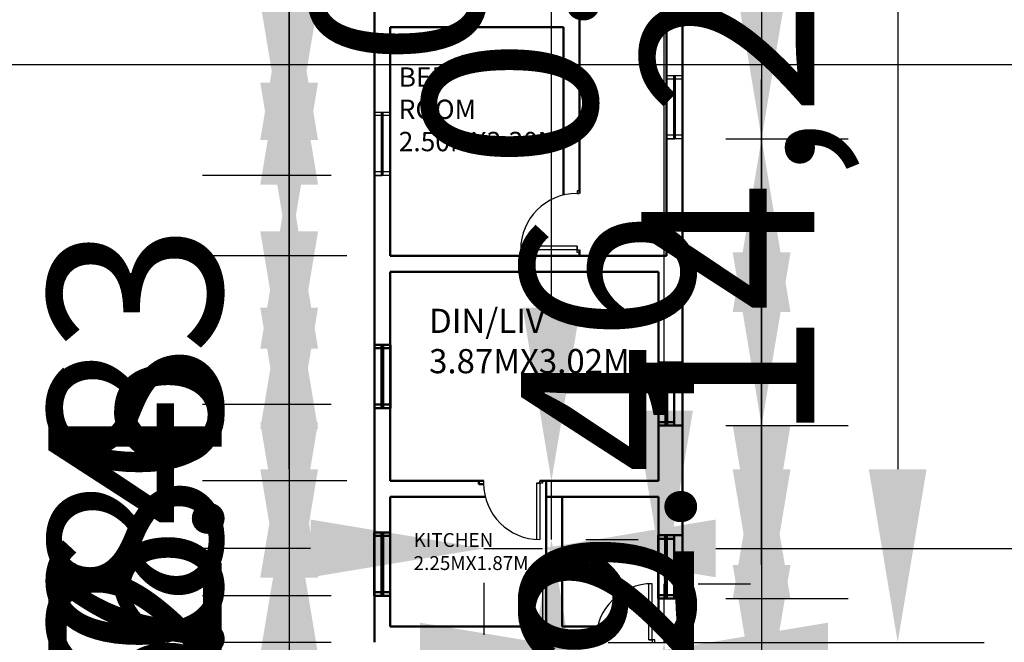
# Model space of a CAD drawing. Units: metres. Extents: x 782 to 1487, y 1262 to 7446.
# Tile 6 of 25: x 807 to 821, y 1293 to 1302. Entities that reach past the tile are written whole.
import ezdxf

# ---------------------------------------------------------------- set-up
doc = ezdxf.new("R2010")
doc.units = ezdxf.units.M
for name, color, linetype, lineweight in [('A-ANNO-DIMS', 2, 'Continuous', 18), ('A-AREA-IDEN', 3, 'Continuous', 18), ('A-DOOR', 4, 'Continuous', 25), ('A-GLAZ', 4, 'Continuous', 25), ('A-WALL', 7, 'Continuous', 50)]:
    doc.layers.add(name, color=color, linetype=linetype, lineweight=lineweight)
doc.styles.get("Standard").update_dxf_attribs({"font": 'arial.ttf'})
doc.dimstyles.new('ISO-25', dxfattribs={"dimtxt": 2.5, "dimasz": 2.5, "dimexe": 1.25, "dimexo": 0.625, "dimtad": 1, "dimtxsty": 'Standard', "dimcen": 2.5, "dimadec": 0, "dimazin": 0, "dimtfac": 1, "dimtmove": 0, "dimatfit": 3, "dimfxl": 1, "dimarcsym": 0})

# ---------------------------------------------------------------- blocks, each defined once
blk = doc.blocks.new('*D4')
at = {"layer": 'A-ANNO-DIMS', "color": 0, "lineweight": -2, "transparency": 16777216}
for p, q in [((817.205, 1307.327), (820.936, 1307.327)), ((819.686, 1304.827), (819.686, 1295.567)), ((817.205, 1293.067), (820.936, 1293.067))]:
    blk.add_line(p, q, dxfattribs=at)
at = {"layer": 'A-ANNO-DIMS', "color": 0, "transparency": 16777216}
for points in [[(819.269, 1304.827), (820.103, 1304.827), (819.686, 1307.327)], [(819.269, 1295.567), (820.103, 1295.567), (819.686, 1293.067)]]:
    blk.add_solid(points, dxfattribs=at)
at = {"layer": 'Defpoints', "color": 0, "transparency": 16777216}
for p in [(816.58, 1307.327), (816.58, 1293.067), (819.686, 1293.067)]:
    blk.add_point(p, dxfattribs=at)
at = {"layer": 'A-ANNO-DIMS', "color": 0, "transparency": 16777216, "insert": (817.558, 1300.197), "char_height": 2.5, "attachment_point": 5, "rotation": 90}
blk.add_mtext('14,26', dxfattribs=at)
blk = doc.blocks.new('DOOR-810')
for p, q in [((0.813, 0.089), (0, 0.089)), ((0.813, 0.038), (0.813, 0.089))]:
    blk.add_line(p, q)
for points in [[(0.813, 0.851), (0.846, 0.851), (0.846, 0.89), (0.813, 0.89)], [(0.813, 0.038), (0.847, 0.038), (0.847, 0), (0.813, 0)]]:
    blk.add_lwpolyline(points, close=True)
blk.add_lwpolyline([(0.813, 0.089), (0.813, 0.038), (0, 0.038)])
blk.add_arc((0.813, 0.038), 0.813, 90, 180)
blk = doc.blocks.new('DOOR-810-B')
for p, q in [((0, 0.813), (0, 0.846)), ((0.812, 0.813), (0.762, 0.813)), ((0.762, 0.813), (0.762, 0))]:
    blk.add_line(p, q)
blk.add_lwpolyline([(0.762, 0.813), (0.812, 0.813), (0.812, 0)])
blk.add_lwpolyline([(0.812, 0.813), (0.812, 0.846), (0.85, 0.846), (0.85, 0.813)], close=True)
blk.add_arc((0.812, 0.813), 0.813, 180, 270)
blk = doc.blocks.new('DOOR-810-C')
for p, q in [((0.801, 0.034), (0.801, 0.847)), ((0.851, 0.034), (0.801, 0.034))]:
    blk.add_line(p, q)
blk.add_lwpolyline([(0.801, 0.034), (0.851, 0.034), (0.851, 0.847)])
for points in [[(0.039, 0.034), (0.039, 0.002), (0, 0.002), (0, 0.034)], [(0.851, 0.034), (0.851, 0), (0.889, 0), (0.889, 0.034)]]:
    blk.add_lwpolyline(points, close=True)
blk.add_arc((0.851, 0.034), 0.813, 90, 180)
blk = doc.blocks.new('WIN-900')
for p, q in [((0, 0), (0, 0.914)), ((0, 0.914), (0.23, 0.914)), ((0.23, 0.863), (0, 0.863)), ((0.102, 0), (0.102, 0.914)), ((0.115, 0), (0.115, 0.914)), ((0.128, 0), (0.128, 0.914)), ((0.23, 0.914), (0.23, 0)), ((0.23, 0.914), (0.23, 0.863)), ((0.23, 0.051), (0, 0.051)), ((0.23, 0), (0.23, 0.051)), ((0.23, 0), (0, 0)), ((0, 0), (0.115, 0))]:
    blk.add_line(p, q)
blk = doc.blocks.new('*D22')
at = {"layer": 'A-ANNO-DIMS', "color": 0, "lineweight": -2, "transparency": 16777216}
for p, q in [((812.79, 1292.934), (810.29, 1292.934)), ((815.29, 1292.934), (816.179, 1292.934)), ((818.679, 1292.934), (848.834, 1292.934)), ((815.29, 1292.442), (815.29, 1291.684)), ((816.179, 1292.442), (816.179, 1291.684))]:
    blk.add_line(p, q, dxfattribs=at)
at = {"layer": 'A-ANNO-DIMS', "color": 0, "transparency": 16777216}
for points in [[(812.79, 1293.351), (812.79, 1292.517), (815.29, 1292.934)], [(818.679, 1293.351), (818.679, 1292.517), (816.179, 1292.934)]]:
    blk.add_solid(points, dxfattribs=at)
at = {"layer": 'Defpoints', "color": 0, "transparency": 16777216}
for p in [(815.29, 1293.067), (816.179, 1293.067), (816.179, 1292.934)]:
    blk.add_point(p, dxfattribs=at)
at = {"layer": 'A-ANNO-DIMS', "color": 0, "transparency": 16777216, "insert": (835.007, 1294.852), "char_height": 2.5, "attachment_point": 5}
blk.add_mtext('DOOR 0.89 TYP.', dxfattribs=at)
blk = doc.blocks.new('*D23')
at = {"layer": 'A-ANNO-DIMS', "color": 0, "lineweight": -2, "transparency": 16777216}
for p, q in [((816.313, 1296.414), (816.313, 1315.246)), ((816.313, 1293.067), (816.313, 1293.914)), ((816.804, 1293.914), (817.563, 1293.914)), ((816.804, 1293.067), (817.563, 1293.067)), ((816.313, 1290.567), (816.313, 1288.067))]:
    blk.add_line(p, q, dxfattribs=at)
at = {"layer": 'A-ANNO-DIMS', "color": 0, "transparency": 16777216}
for points in [[(815.896, 1296.414), (816.729, 1296.414), (816.313, 1293.914)], [(815.896, 1290.567), (816.729, 1290.567), (816.313, 1293.067)]]:
    blk.add_solid(points, dxfattribs=at)
at = {"layer": 'Defpoints', "color": 0, "transparency": 16777216}
for p in [(816.179, 1293.914), (816.313, 1293.914), (816.179, 1293.067)]:
    blk.add_point(p, dxfattribs=at)
at = {"layer": 'A-ANNO-DIMS', "color": 0, "transparency": 16777216, "insert": (814.411, 1307.08), "char_height": 2.5, "attachment_point": 5, "rotation": 90}
blk.add_mtext('0.85 TYP.', dxfattribs=at)
blk = doc.blocks.new('*D24')
at = {"layer": 'A-ANNO-DIMS', "color": 0, "lineweight": -2, "transparency": 16777216}
for p, q in [((811.209, 1294.423), (808.709, 1294.423)), ((813.709, 1294.423), (814.559, 1294.423)), ((817.059, 1294.423), (852.649, 1294.423)), ((813.709, 1293.926), (813.709, 1293.173)), ((814.559, 1293.926), (814.559, 1293.173))]:
    blk.add_line(p, q, dxfattribs=at)
at = {"layer": 'A-ANNO-DIMS', "color": 0, "transparency": 16777216}
for points in [[(811.209, 1294.84), (811.209, 1294.006), (813.709, 1294.423)], [(817.059, 1294.84), (817.059, 1294.006), (814.559, 1294.423)]]:
    blk.add_solid(points, dxfattribs=at)
at = {"layer": 'Defpoints', "color": 0, "transparency": 16777216}
for p in [(813.709, 1294.551), (814.559, 1294.551), (814.559, 1294.423)]:
    blk.add_point(p, dxfattribs=at)
at = {"layer": 'A-ANNO-DIMS', "color": 0, "transparency": 16777216, "insert": (836.104, 1296.342), "char_height": 2.5, "attachment_point": 5}
blk.add_mtext('DOOR D2 0.85 TYP.', dxfattribs=at)
blk = doc.blocks.new('*D25')
at = {"layer": 'A-ANNO-DIMS', "color": 0, "lineweight": -2, "transparency": 16777216}
for p, q in [((814.687, 1297.897), (814.687, 1316.729)), ((814.687, 1294.551), (814.687, 1295.397)), ((815.184, 1295.397), (815.937, 1295.397)), ((815.184, 1294.551), (815.937, 1294.551)), ((814.687, 1292.051), (814.687, 1289.551))]:
    blk.add_line(p, q, dxfattribs=at)
at = {"layer": 'A-ANNO-DIMS', "color": 0, "transparency": 16777216}
for points in [[(814.27, 1297.897), (815.103, 1297.897), (814.687, 1295.397)], [(814.27, 1292.051), (815.103, 1292.051), (814.687, 1294.551)]]:
    blk.add_solid(points, dxfattribs=at)
at = {"layer": 'Defpoints', "color": 0, "transparency": 16777216}
for p in [(814.559, 1295.397), (814.687, 1295.397), (814.559, 1294.551)]:
    blk.add_point(p, dxfattribs=at)
at = {"layer": 'A-ANNO-DIMS', "color": 0, "transparency": 16777216, "insert": (812.785, 1308.563), "char_height": 2.5, "attachment_point": 5, "rotation": 90}
blk.add_mtext('0.85 TYP.', dxfattribs=at)
blk = doc.blocks.new('*D26')
at = {"layer": 'A-ANNO-DIMS', "color": 0, "lineweight": -2, "transparency": 16777216}
for p, q in [((828.33, 1303.223), (828.33, 1342.718)), ((828.33, 1299.809), (828.33, 1300.723)), ((828.818, 1300.723), (829.58, 1300.723)), ((828.818, 1299.809), (829.58, 1299.809)), ((828.33, 1297.309), (828.33, 1294.809))]:
    blk.add_line(p, q, dxfattribs=at)
at = {"layer": 'A-ANNO-DIMS', "color": 0, "transparency": 16777216}
for points in [[(827.913, 1303.223), (828.747, 1303.223), (828.33, 1300.723)], [(827.913, 1297.309), (828.747, 1297.309), (828.33, 1299.809)]]:
    blk.add_solid(points, dxfattribs=at)
at = {"layer": 'Defpoints', "color": 0, "transparency": 16777216}
for p in [(828.193, 1300.723), (828.33, 1300.723), (828.193, 1299.809)]:
    blk.add_point(p, dxfattribs=at)
at = {"layer": 'A-ANNO-DIMS', "color": 0, "transparency": 16777216, "insert": (826.412, 1324.22), "char_height": 2.5, "attachment_point": 5, "rotation": 90}
blk.add_mtext('WINDOW W 0.91 TYP.', dxfattribs=at)
blk = doc.blocks.new('*D30')
at = {"layer": 'A-ANNO-DIMS', "color": 0, "lineweight": -2, "transparency": 16777216}
for p, q in [((792.059, 1301.411), (789.559, 1301.411)), ((794.559, 1301.411), (794.946, 1301.411)), ((797.446, 1301.411), (832.354, 1301.411)), ((794.559, 1300.844), (794.559, 1300.161)), ((794.946, 1300.844), (794.946, 1300.161))]:
    blk.add_line(p, q, dxfattribs=at)
at = {"layer": 'A-ANNO-DIMS', "color": 0, "transparency": 16777216}
for points in [[(792.059, 1301.827), (792.059, 1300.994), (794.559, 1301.411)], [(797.446, 1301.827), (797.446, 1300.994), (794.946, 1301.411)]]:
    blk.add_solid(points, dxfattribs=at)
at = {"layer": 'Defpoints', "color": 0, "transparency": 16777216}
for p in [(794.559, 1301.469), (794.946, 1301.469), (794.946, 1301.411)]:
    blk.add_point(p, dxfattribs=at)
at = {"layer": 'A-ANNO-DIMS', "color": 0, "transparency": 16777216, "insert": (816.15, 1303.33), "char_height": 2.5, "attachment_point": 5}
blk.add_mtext('COLUMN 0.39 TYP.', dxfattribs=at)
blk = doc.blocks.new('*D48')
at = {"layer": 'A-ANNO-DIMS', "color": 0, "lineweight": -2, "transparency": 16777216}
for p, q in [((795.937, 1293.455), (795.937, 1287.89)), ((794.559, 1292.035), (794.559, 1287.89)), ((792.059, 1289.14), (789.559, 1289.14)), ((794.559, 1289.14), (795.937, 1289.14)), ((798.437, 1289.14), (808.45, 1289.14))]:
    blk.add_line(p, q, dxfattribs=at)
at = {"layer": 'A-ANNO-DIMS', "color": 0, "transparency": 16777216}
for points in [[(792.059, 1289.557), (792.059, 1288.724), (794.559, 1289.14)], [(798.437, 1289.557), (798.437, 1288.724), (795.937, 1289.14)]]:
    blk.add_solid(points, dxfattribs=at)
at = {"layer": 'Defpoints', "color": 0, "transparency": 16777216}
for p in [(795.937, 1294.08), (794.559, 1292.66), (795.937, 1289.14)]:
    blk.add_point(p, dxfattribs=at)
at = {"layer": 'A-ANNO-DIMS', "color": 0, "transparency": 16777216, "insert": (804.694, 1291.043), "char_height": 2.5, "attachment_point": 5}
blk.add_mtext('1.38', dxfattribs=at)
blk = doc.blocks.new('*D53')
at = {"layer": 'A-ANNO-DIMS', "color": 0, "lineweight": -2, "transparency": 16777216}
for p, q in [((810.9, 1309.827), (810.9, 1312.327)), ((811.505, 1307.327), (809.65, 1307.327)), ((810.9, 1307.327), (810.9, 1304.697)), ((811.735, 1304.697), (809.65, 1304.697)), ((810.9, 1302.197), (810.9, 1291.911))]:
    blk.add_line(p, q, dxfattribs=at)
at = {"layer": 'A-ANNO-DIMS', "color": 0, "transparency": 16777216}
for points in [[(810.483, 1309.827), (811.317, 1309.827), (810.9, 1307.327)], [(810.483, 1302.197), (811.317, 1302.197), (810.9, 1304.697)]]:
    blk.add_solid(points, dxfattribs=at)
at = {"layer": 'Defpoints', "color": 0, "transparency": 16777216}
for p in [(812.13, 1307.327), (810.9, 1304.697), (812.36, 1304.697)]:
    blk.add_point(p, dxfattribs=at)
at = {"layer": 'A-ANNO-DIMS', "color": 0, "transparency": 16777216, "insert": (808.998, 1295.804), "char_height": 2.5, "attachment_point": 5, "rotation": 90}
blk.add_mtext('2.63', dxfattribs=at)
blk = doc.blocks.new('*D54')
at = {"layer": 'A-ANNO-DIMS', "color": 0, "lineweight": -2, "transparency": 16777216}
for p, q in [((810.9, 1307.197), (810.9, 1309.697)), ((811.735, 1304.697), (809.65, 1304.697)), ((810.9, 1304.697), (810.9, 1302.822)), ((811.503, 1302.822), (809.65, 1302.822)), ((810.9, 1300.322), (810.9, 1290.308))]:
    blk.add_line(p, q, dxfattribs=at)
at = {"layer": 'A-ANNO-DIMS', "color": 0, "transparency": 16777216}
for points in [[(810.483, 1307.197), (811.317, 1307.197), (810.9, 1304.697)], [(810.483, 1300.322), (811.317, 1300.322), (810.9, 1302.822)]]:
    blk.add_solid(points, dxfattribs=at)
at = {"layer": 'Defpoints', "color": 0, "transparency": 16777216}
for p in [(812.36, 1304.697), (810.9, 1302.822), (812.128, 1302.822)]:
    blk.add_point(p, dxfattribs=at)
at = {"layer": 'A-ANNO-DIMS', "color": 0, "transparency": 16777216, "insert": (808.999, 1294.065), "char_height": 2.5, "attachment_point": 5, "rotation": 90}
blk.add_mtext('1.88', dxfattribs=at)
blk = doc.blocks.new('*D55')
at = {"layer": 'A-ANNO-DIMS', "color": 0, "lineweight": -2, "transparency": 16777216}
for p, q in [((810.9, 1305.322), (810.9, 1307.822)), ((811.503, 1302.822), (809.65, 1302.822)), ((810.9, 1302.822), (810.9, 1302.177)), ((811.735, 1302.177), (809.65, 1302.177)), ((810.9, 1299.677), (810.9, 1289.444))]:
    blk.add_line(p, q, dxfattribs=at)
at = {"layer": 'A-ANNO-DIMS', "color": 0, "transparency": 16777216}
for points in [[(810.483, 1305.322), (811.317, 1305.322), (810.9, 1302.822)], [(810.483, 1299.677), (811.317, 1299.677), (810.9, 1302.177)]]:
    blk.add_solid(points, dxfattribs=at)
at = {"layer": 'Defpoints', "color": 0, "transparency": 16777216}
for p in [(812.128, 1302.822), (810.9, 1302.177), (812.36, 1302.177)]:
    blk.add_point(p, dxfattribs=at)
at = {"layer": 'A-ANNO-DIMS', "color": 0, "transparency": 16777216, "insert": (808.999, 1293.311), "char_height": 2.5, "attachment_point": 5, "rotation": 90}
blk.add_mtext('0.64', dxfattribs=at)
blk = doc.blocks.new('*D56')
at = {"layer": 'A-ANNO-DIMS', "color": 0, "lineweight": -2, "transparency": 16777216}
for p, q in [((810.9, 1304.677), (810.9, 1307.177)), ((811.735, 1302.177), (809.65, 1302.177)), ((810.9, 1302.177), (810.9, 1299.809)), ((811.505, 1299.809), (809.65, 1299.809)), ((810.9, 1297.309), (810.9, 1287.022))]:
    blk.add_line(p, q, dxfattribs=at)
at = {"layer": 'A-ANNO-DIMS', "color": 0, "transparency": 16777216}
for points in [[(810.483, 1304.677), (811.317, 1304.677), (810.9, 1302.177)], [(810.483, 1297.309), (811.317, 1297.309), (810.9, 1299.809)]]:
    blk.add_solid(points, dxfattribs=at)
at = {"layer": 'Defpoints', "color": 0, "transparency": 16777216}
for p in [(812.36, 1302.177), (810.9, 1299.809), (812.13, 1299.809)]:
    blk.add_point(p, dxfattribs=at)
at = {"layer": 'A-ANNO-DIMS', "color": 0, "transparency": 16777216, "insert": (808.998, 1290.916), "char_height": 2.5, "attachment_point": 5, "rotation": 90}
blk.add_mtext('2.37', dxfattribs=at)
blk = doc.blocks.new('*D57')
at = {"layer": 'A-ANNO-DIMS', "color": 0, "lineweight": -2, "transparency": 16777216}
for p, q in [((810.9, 1302.309), (810.9, 1304.809)), ((811.505, 1299.809), (809.65, 1299.809)), ((810.9, 1299.809), (810.9, 1298.647)), ((811.735, 1298.647), (809.65, 1298.647)), ((810.9, 1296.147), (810.9, 1286.141))]:
    blk.add_line(p, q, dxfattribs=at)
at = {"layer": 'A-ANNO-DIMS', "color": 0, "transparency": 16777216}
for points in [[(810.483, 1302.309), (811.317, 1302.309), (810.9, 1299.809)], [(810.483, 1296.147), (811.317, 1296.147), (810.9, 1298.647)]]:
    blk.add_solid(points, dxfattribs=at)
at = {"layer": 'Defpoints', "color": 0, "transparency": 16777216}
for p in [(812.13, 1299.809), (810.9, 1298.647), (812.36, 1298.647)]:
    blk.add_point(p, dxfattribs=at)
at = {"layer": 'A-ANNO-DIMS', "color": 0, "transparency": 16777216, "insert": (808.999, 1289.894), "char_height": 2.5, "attachment_point": 5, "rotation": 90}
blk.add_mtext('1.16', dxfattribs=at)
blk = doc.blocks.new('*D58')
at = {"layer": 'A-ANNO-DIMS', "color": 0, "lineweight": -2, "transparency": 16777216}
for p, q in [((810.9, 1301.147), (810.9, 1303.647)), ((811.735, 1298.647), (809.65, 1298.647)), ((810.9, 1298.647), (810.9, 1296.5)), ((811.507, 1296.5), (809.65, 1296.5)), ((810.9, 1294), (810.9, 1281.772))]:
    blk.add_line(p, q, dxfattribs=at)
at = {"layer": 'A-ANNO-DIMS', "color": 0, "transparency": 16777216}
for points in [[(810.483, 1301.147), (811.317, 1301.147), (810.9, 1298.647)], [(810.483, 1294), (811.317, 1294), (810.9, 1296.5)]]:
    blk.add_solid(points, dxfattribs=at)
at = {"layer": 'Defpoints', "color": 0, "transparency": 16777216}
for p in [(812.36, 1298.647), (810.9, 1296.5), (812.132, 1296.5)]:
    blk.add_point(p, dxfattribs=at)
at = {"layer": 'A-ANNO-DIMS', "color": 0, "transparency": 16777216, "insert": (809.02, 1286.636), "char_height": 2.5, "attachment_point": 5, "rotation": 90}
blk.add_mtext('2.147', dxfattribs=at)
blk = doc.blocks.new('*D59')
at = {"layer": 'A-ANNO-DIMS', "color": 0, "lineweight": -2, "transparency": 16777216}
for p, q in [((810.9, 1299), (810.9, 1301.5)), ((811.507, 1296.5), (809.65, 1296.5)), ((810.9, 1296.5), (810.9, 1295.397)), ((811.735, 1295.397), (809.65, 1295.397)), ((810.9, 1292.897), (810.9, 1280.947))]:
    blk.add_line(p, q, dxfattribs=at)
at = {"layer": 'A-ANNO-DIMS', "color": 0, "transparency": 16777216}
for points in [[(810.483, 1299), (811.317, 1299), (810.9, 1296.5)], [(810.483, 1292.897), (811.317, 1292.897), (810.9, 1295.397)]]:
    blk.add_solid(points, dxfattribs=at)
at = {"layer": 'Defpoints', "color": 0, "transparency": 16777216}
for p in [(812.132, 1296.5), (810.9, 1295.397), (812.36, 1295.397)]:
    blk.add_point(p, dxfattribs=at)
at = {"layer": 'A-ANNO-DIMS', "color": 0, "transparency": 16777216, "insert": (808.998, 1285.672), "char_height": 2.5, "attachment_point": 5, "rotation": 90}
blk.add_mtext('1.103', dxfattribs=at)
blk = doc.blocks.new('*D60')
at = {"layer": 'A-ANNO-DIMS', "color": 0, "lineweight": -2, "transparency": 16777216}
for p, q in [((810.9, 1297.897), (810.9, 1300.397)), ((811.735, 1295.397), (809.65, 1295.397)), ((810.9, 1295.397), (810.9, 1293.74)), ((811.505, 1293.74), (809.65, 1293.74)), ((810.9, 1291.24), (810.9, 1281.233))]:
    blk.add_line(p, q, dxfattribs=at)
at = {"layer": 'A-ANNO-DIMS', "color": 0, "transparency": 16777216}
for points in [[(810.483, 1297.897), (811.317, 1297.897), (810.9, 1295.397)], [(810.483, 1291.24), (811.317, 1291.24), (810.9, 1293.74)]]:
    blk.add_solid(points, dxfattribs=at)
at = {"layer": 'Defpoints', "color": 0, "transparency": 16777216}
for p in [(812.36, 1295.397), (810.9, 1293.74), (812.13, 1293.74)]:
    blk.add_point(p, dxfattribs=at)
at = {"layer": 'A-ANNO-DIMS', "color": 0, "transparency": 16777216, "insert": (808.999, 1284.987), "char_height": 2.5, "attachment_point": 5, "rotation": 90}
blk.add_mtext('1.66', dxfattribs=at)
blk = doc.blocks.new('*D61')
at = {"layer": 'A-ANNO-DIMS', "color": 0, "lineweight": -2, "transparency": 16777216}
for p, q in [((810.9, 1296.24), (810.9, 1298.74)), ((811.505, 1293.74), (809.65, 1293.74)), ((810.9, 1293.74), (810.9, 1293.067)), ((811.505, 1293.067), (809.65, 1293.067)), ((810.9, 1290.567), (810.9, 1280.324))]:
    blk.add_line(p, q, dxfattribs=at)
at = {"layer": 'A-ANNO-DIMS', "color": 0, "transparency": 16777216}
for points in [[(810.483, 1296.24), (811.317, 1296.24), (810.9, 1293.74)], [(810.483, 1290.567), (811.317, 1290.567), (810.9, 1293.067)]]:
    blk.add_solid(points, dxfattribs=at)
at = {"layer": 'Defpoints', "color": 0, "transparency": 16777216}
for p in [(812.13, 1293.74), (810.9, 1293.067), (812.13, 1293.067)]:
    blk.add_point(p, dxfattribs=at)
at = {"layer": 'A-ANNO-DIMS', "color": 0, "transparency": 16777216, "insert": (808.999, 1284.195), "char_height": 2.5, "attachment_point": 5, "rotation": 90}
blk.add_mtext('0.67', dxfattribs=at)
blk = doc.blocks.new('*D62')
at = {"layer": 'A-ANNO-DIMS', "color": 0, "lineweight": -2, "transparency": 16777216}
for p, q in [((810.9, 1295.567), (810.9, 1298.067)), ((811.505, 1293.067), (809.65, 1293.067)), ((810.9, 1293.067), (810.9, 1290.305)), ((811.505, 1290.305), (809.65, 1290.305)), ((810.9, 1287.805), (810.9, 1275.602))]:
    blk.add_line(p, q, dxfattribs=at)
at = {"layer": 'A-ANNO-DIMS', "color": 0, "transparency": 16777216}
for points in [[(810.483, 1295.567), (811.317, 1295.567), (810.9, 1293.067)], [(810.483, 1287.805), (811.317, 1287.805), (810.9, 1290.305)]]:
    blk.add_solid(points, dxfattribs=at)
at = {"layer": 'Defpoints', "color": 0, "transparency": 16777216}
for p in [(812.13, 1293.067), (810.9, 1290.305), (812.13, 1290.305)]:
    blk.add_point(p, dxfattribs=at)
at = {"layer": 'A-ANNO-DIMS', "color": 0, "transparency": 16777216, "insert": (808.999, 1280.454), "char_height": 2.5, "attachment_point": 5, "rotation": 90}
blk.add_mtext('2.762', dxfattribs=at)
blk = doc.blocks.new('*D63')
at = {"layer": 'A-ANNO-DIMS', "color": 0, "lineweight": -2, "transparency": 16777216}
for p, q in [((817.721, 1309.827), (817.721, 1312.327)), ((817.205, 1307.327), (818.971, 1307.327)), ((817.721, 1307.327), (817.721, 1304.867)), ((817.205, 1304.867), (818.971, 1304.867)), ((817.721, 1302.367), (817.721, 1292.082))]:
    blk.add_line(p, q, dxfattribs=at)
at = {"layer": 'A-ANNO-DIMS', "color": 0, "transparency": 16777216}
for points in [[(817.304, 1309.827), (818.138, 1309.827), (817.721, 1307.327)], [(817.304, 1302.367), (818.138, 1302.367), (817.721, 1304.867)]]:
    blk.add_solid(points, dxfattribs=at)
at = {"layer": 'Defpoints', "color": 0, "transparency": 16777216}
for p in [(816.58, 1307.327), (816.58, 1304.867), (817.721, 1304.867)]:
    blk.add_point(p, dxfattribs=at)
at = {"layer": 'A-ANNO-DIMS', "color": 0, "transparency": 16777216, "insert": (815.82, 1295.974), "char_height": 2.5, "attachment_point": 5, "rotation": 90}
blk.add_mtext('2.46', dxfattribs=at)
blk = doc.blocks.new('*D64')
at = {"layer": 'A-ANNO-DIMS', "color": 0, "lineweight": -2, "transparency": 16777216}
for p, q in [((817.721, 1307.367), (817.721, 1309.867)), ((817.205, 1304.867), (818.971, 1304.867)), ((817.721, 1304.867), (817.721, 1300.338)), ((817.206, 1300.338), (818.971, 1300.338)), ((817.721, 1297.838), (817.721, 1285.546))]:
    blk.add_line(p, q, dxfattribs=at)
at = {"layer": 'A-ANNO-DIMS', "color": 0, "transparency": 16777216}
for points in [[(817.304, 1307.367), (818.138, 1307.367), (817.721, 1304.867)], [(817.304, 1297.838), (818.138, 1297.838), (817.721, 1300.338)]]:
    blk.add_solid(points, dxfattribs=at)
at = {"layer": 'Defpoints', "color": 0, "transparency": 16777216}
for p in [(816.58, 1304.867), (816.581, 1300.338), (817.721, 1300.338)]:
    blk.add_point(p, dxfattribs=at)
at = {"layer": 'A-ANNO-DIMS', "color": 0, "transparency": 16777216, "insert": (815.82, 1290.442), "char_height": 2.5, "attachment_point": 5, "rotation": 90}
blk.add_mtext('4.529', dxfattribs=at)
blk = doc.blocks.new('*D65')
at = {"layer": 'A-ANNO-DIMS', "color": 0, "lineweight": -2, "transparency": 16777216}
for p, q in [((817.721, 1302.838), (817.721, 1305.338)), ((817.206, 1300.338), (818.971, 1300.338)), ((817.721, 1300.338), (817.721, 1296.196)), ((817.205, 1296.196), (818.971, 1296.196)), ((817.721, 1293.696), (817.721, 1281.435))]:
    blk.add_line(p, q, dxfattribs=at)
at = {"layer": 'A-ANNO-DIMS', "color": 0, "transparency": 16777216}
for points in [[(817.304, 1302.838), (818.138, 1302.838), (817.721, 1300.338)], [(817.304, 1293.696), (818.138, 1293.696), (817.721, 1296.196)]]:
    blk.add_solid(points, dxfattribs=at)
at = {"layer": 'Defpoints', "color": 0, "transparency": 16777216}
for p in [(816.581, 1300.338), (816.58, 1296.196), (817.721, 1296.196)]:
    blk.add_point(p, dxfattribs=at)
at = {"layer": 'A-ANNO-DIMS', "color": 0, "transparency": 16777216, "insert": (815.841, 1286.315), "char_height": 2.5, "attachment_point": 5, "rotation": 90}
blk.add_mtext('4.142', dxfattribs=at)
blk = doc.blocks.new('*D66')
at = {"layer": 'A-ANNO-DIMS', "color": 0, "lineweight": -2, "transparency": 16777216}
for p, q in [((817.721, 1298.696), (817.721, 1301.196)), ((817.205, 1296.196), (818.971, 1296.196)), ((817.721, 1296.196), (817.721, 1293.699)), ((817.205, 1293.699), (818.971, 1293.699)), ((817.721, 1291.199), (817.721, 1280.921))]:
    blk.add_line(p, q, dxfattribs=at)
at = {"layer": 'A-ANNO-DIMS', "color": 0, "transparency": 16777216}
for points in [[(817.304, 1298.696), (818.138, 1298.696), (817.721, 1296.196)], [(817.304, 1291.199), (818.138, 1291.199), (817.721, 1293.699)]]:
    blk.add_solid(points, dxfattribs=at)
at = {"layer": 'Defpoints', "color": 0, "transparency": 16777216}
for p in [(816.58, 1296.196), (816.58, 1293.699), (817.721, 1293.699)]:
    blk.add_point(p, dxfattribs=at)
at = {"layer": 'A-ANNO-DIMS', "color": 0, "transparency": 16777216, "insert": (815.82, 1284.81), "char_height": 2.5, "attachment_point": 5, "rotation": 90}
blk.add_mtext('2.50', dxfattribs=at)
blk = doc.blocks.new('*D67')
at = {"layer": 'A-ANNO-DIMS', "color": 0, "lineweight": -2, "transparency": 16777216}
for p, q in [((817.721, 1296.199), (817.721, 1298.699)), ((817.205, 1293.699), (818.971, 1293.699)), ((817.721, 1293.699), (817.721, 1293.067)), ((817.205, 1293.067), (818.971, 1293.067)), ((817.721, 1290.567), (817.721, 1278.407))]:
    blk.add_line(p, q, dxfattribs=at)
at = {"layer": 'A-ANNO-DIMS', "color": 0, "transparency": 16777216}
for points in [[(817.304, 1296.199), (818.138, 1296.199), (817.721, 1293.699)], [(817.304, 1290.567), (818.138, 1290.567), (817.721, 1293.067)]]:
    blk.add_solid(points, dxfattribs=at)
at = {"layer": 'Defpoints', "color": 0, "transparency": 16777216}
for p in [(816.58, 1293.699), (816.58, 1293.067), (817.721, 1293.067)]:
    blk.add_point(p, dxfattribs=at)
at = {"layer": 'A-ANNO-DIMS', "color": 0, "transparency": 16777216, "insert": (815.819, 1283.237), "char_height": 2.5, "attachment_point": 5, "rotation": 90}
blk.add_mtext('0.632', dxfattribs=at)
blk = doc.blocks.new('*D68')
at = {"layer": 'A-ANNO-DIMS', "color": 0, "lineweight": -2, "transparency": 16777216}
for p, q in [((817.721, 1295.567), (817.721, 1298.067)), ((815.508, 1293.067), (818.971, 1293.067)), ((817.721, 1293.067), (817.721, 1291.686)), ((815.508, 1291.686), (818.971, 1291.686)), ((817.721, 1289.186), (817.721, 1277.718))]:
    blk.add_line(p, q, dxfattribs=at)
at = {"layer": 'A-ANNO-DIMS', "color": 0, "transparency": 16777216}
for points in [[(817.304, 1295.567), (818.138, 1295.567), (817.721, 1293.067)], [(817.304, 1289.186), (818.138, 1289.186), (817.721, 1291.686)]]:
    blk.add_solid(points, dxfattribs=at)
at = {"layer": 'Defpoints', "color": 0, "transparency": 16777216}
for p in [(814.883, 1293.067), (814.883, 1291.686), (817.721, 1291.686)]:
    blk.add_point(p, dxfattribs=at)
at = {"layer": 'A-ANNO-DIMS', "color": 0, "transparency": 16777216, "insert": (815.819, 1282.202), "char_height": 2.5, "attachment_point": 5, "rotation": 90}
blk.add_mtext('1.381', dxfattribs=at)
blk = doc.blocks.new('*D69')
at = {"layer": 'A-ANNO-DIMS', "color": 0, "lineweight": -2, "transparency": 16777216}
for p, q in [((817.721, 1294.186), (817.721, 1296.686)), ((815.508, 1291.686), (818.971, 1291.686)), ((817.721, 1291.686), (817.721, 1290.305)), ((815.508, 1290.305), (818.971, 1290.305)), ((817.721, 1287.805), (817.721, 1276.337))]:
    blk.add_line(p, q, dxfattribs=at)
at = {"layer": 'A-ANNO-DIMS', "color": 0, "transparency": 16777216}
for points in [[(817.304, 1294.186), (818.138, 1294.186), (817.721, 1291.686)], [(817.304, 1287.805), (818.138, 1287.805), (817.721, 1290.305)]]:
    blk.add_solid(points, dxfattribs=at)
at = {"layer": 'Defpoints', "color": 0, "transparency": 16777216}
for p in [(814.883, 1291.686), (814.883, 1290.305), (817.721, 1290.305)]:
    blk.add_point(p, dxfattribs=at)
at = {"layer": 'A-ANNO-DIMS', "color": 0, "transparency": 16777216, "insert": (815.819, 1280.821), "char_height": 2.5, "attachment_point": 5, "rotation": 90}
blk.add_mtext('1.381', dxfattribs=at)

msp = doc.modelspace()

# ---------------------------------------------------------------- linework, layer by layer
at = {"layer": 'A-WALL'}
for p, q in [((816.58, 1303.3374), (816.58, 1293.0674)), ((816.35, 1303.1074), (816.35, 1298.6474)), ((812.13, 1298.6474), (812.13, 1302.1774)), ((815.09, 1302.1774), (815.09, 1299.5481)), ((812.36, 1298.6474), (812.36, 1301.9474)), ((812.36, 1301.9474), (814.86, 1301.9474)), ((814.86, 1301.9474), (814.86, 1299.5248)), ((815.09, 1298.736), (815.09, 1298.6474)), ((812.13, 1295.3974), (812.13, 1298.6474)), ((812.36, 1298.6474), (816.23, 1298.6474)), ((815.09, 1298.6474), (815.09, 1298.6982)), ((816.35, 1298.6474), (816.23, 1298.6474)), ((812.36, 1295.3974), (812.36, 1298.4174)), ((812.36, 1298.4174), (816.23, 1298.4174)), ((812.36, 1298.4174), (816.23, 1298.4174)), ((816.23, 1298.4174), (816.23, 1295.3974)), ((812.1317, 1296.4496), (812.1317, 1297.3636)), ((812.1317, 1297.3636), (812.3617, 1297.3636)), ((812.3617, 1297.3128), (812.1317, 1297.3128)), ((812.234, 1296.4496), (812.234, 1297.3636)), ((812.2467, 1296.4496), (812.2467, 1297.3636)), ((812.2594, 1296.4496), (812.2594, 1297.3636)), ((812.3617, 1297.3636), (812.3617, 1296.4496)), ((812.3617, 1297.3636), (812.3617, 1297.3128)), ((816.2301, 1296.196), (816.2301, 1297.11)), ((816.2301, 1297.11), (816.4601, 1297.11)), ((816.4601, 1297.0592), (816.2301, 1297.0592)), ((816.3324, 1296.196), (816.3324, 1297.11)), ((816.3451, 1296.196), (816.3451, 1297.11)), ((816.3578, 1296.196), (816.3578, 1297.11)), ((816.4601, 1297.11), (816.4601, 1296.196)), ((816.4601, 1297.11), (816.4601, 1297.0592)), ((816.4601, 1297.11), (816.58, 1297.11)), ((816.58, 1297.11), (816.58, 1296.196)), ((812.3617, 1296.5004), (812.1317, 1296.5004)), ((812.3617, 1296.4496), (812.3617, 1296.5004)), ((812.3617, 1296.4496), (812.1317, 1296.4496)), ((812.1317, 1296.4496), (812.2467, 1296.4496)), ((816.4601, 1296.2468), (816.2301, 1296.2468)), ((816.4601, 1296.196), (816.2301, 1296.196)), ((816.2301, 1296.196), (816.3451, 1296.196)), ((816.4601, 1296.196), (816.4601, 1296.2468)), ((816.58, 1296.196), (816.4601, 1296.196)), ((812.13, 1295.3974), (812.13, 1293.0674)), ((813.7093, 1295.3974), (812.36, 1295.3974)), ((813.7093, 1295.3974), (812.36, 1295.3974)), ((813.7086, 1295.3974), (813.6406, 1295.3974)), ((813.6406, 1295.3974), (813.6406, 1295.3502)), ((813.6406, 1295.3502), (813.7087, 1295.3502)), ((814.61, 1295.3974), (814.5214, 1295.3974)), ((816.23, 1295.3974), (814.5214, 1295.3974)), ((814.61, 1295.3974), (814.5592, 1295.3974)), ((814.61, 1295.1674), (814.61, 1295.3974)), ((812.36, 1295.1674), (812.36, 1293.2974)), ((813.7326, 1295.1674), (812.36, 1295.1674)), ((813.7326, 1295.1674), (812.36, 1295.1674)), ((814.61, 1293.2974), (814.61, 1295.1674)), ((816.23, 1295.1674), (814.61, 1295.1674)), ((814.84, 1293.2974), (814.84, 1295.1674)), ((816.23, 1293.2974), (816.23, 1295.1674)), ((812.1297, 1293.7402), (812.1297, 1294.6542)), ((812.1297, 1294.6542), (812.3597, 1294.6542)), ((812.232, 1293.7402), (812.232, 1294.6542)), ((812.2447, 1293.7402), (812.2447, 1294.6542)), ((812.2574, 1293.7402), (812.2574, 1294.6542)), ((812.3597, 1294.6542), (812.3597, 1293.7402)), ((812.3597, 1294.6542), (812.3597, 1294.6034)), ((816.2268, 1293.6994), (816.2268, 1294.6134)), ((816.2268, 1294.6134), (816.4568, 1294.6134)), ((816.3291, 1293.6994), (816.3291, 1294.6134)), ((816.3418, 1293.6994), (816.3418, 1294.6134)), ((816.3545, 1293.6994), (816.3545, 1294.6134)), ((816.4568, 1294.6134), (816.4568, 1293.6994)), ((816.4568, 1294.6134), (816.4568, 1294.5626)), ((816.4568, 1294.6134), (816.58, 1294.6134)), ((816.58, 1294.6134), (816.58, 1293.6994)), ((812.3597, 1294.6034), (812.1297, 1294.6034)), ((816.4568, 1294.5626), (816.2268, 1294.5626)), ((812.3597, 1293.791), (812.1297, 1293.791)), ((812.3597, 1293.7402), (812.3597, 1293.791)), ((812.3597, 1293.7402), (812.1297, 1293.7402)), ((812.1297, 1293.7402), (812.2447, 1293.7402)), ((816.4568, 1293.7502), (816.2268, 1293.7502)), ((816.4568, 1293.6994), (816.2268, 1293.6994)), ((816.2268, 1293.6994), (816.3418, 1293.6994)), ((816.4568, 1293.6994), (816.4568, 1293.7502)), ((816.58, 1293.6994), (816.4568, 1293.6994)), ((812.36, 1293.2974), (814.61, 1293.2974)), ((814.84, 1293.2974), (815.3526, 1293.2974)), ((816.1414, 1293.2974), (816.23, 1293.2974))]:
    msp.add_line(p, q, dxfattribs=at)

# ---------------------------------------------------------------- block references
at = {"layer": 'A-DOOR'}
for name, p in [('DOOR-810', (814.243, 1298.698)), ('DOOR-810-B', (813.709, 1294.551)), ('DOOR-810-C', (815.29, 1293.067))]:
    msp.add_blockref(name, p, dxfattribs=at)
at = {"layer": 'A-GLAZ'}
for p in [(816.351, 1300.338), (812.13, 1299.809)]:
    msp.add_blockref('WIN-900', p, dxfattribs=at)

# ---------------------------------------------------------------- texts
at = {"layer": 'A-AREA-IDEN', "attachment_point": 1}
for s, width, gutter_width, insert, char_height in [('BED ROOM\\P2.50MX3.30M', 0.64421, 6.9836, (812.4812, 1301.3688), 0.279342), ('DIN/LIV\\P3.87MX3.02M', 0.805163, 8.7284, (812.9207, 1297.8835), 0.349134), ('{\\H0.4x;\\PKITCHEN\\P2.25MX1.87M}', 1.153085, 12.5, (812.6969, 1294.9782), 0.5)]:
    msp.add_mtext_dynamic_manual_height_columns(s, width=width, gutter_width=gutter_width, heights=[0], dxfattribs=dict(at, insert=insert, char_height=char_height))

# ---------------------------------------------------------------- dimensions: what is measured, and where the dimension line sits
at = {"layer": 'A-ANNO-DIMS'}
for base, p1, p2, text, picture, middle in [((828.3302, 1300.7228), (828.1931, 1299.8088), (828.1931, 1300.7228), 'WINDOW W <> TYP.', '*D26', (826.4117, 1324.2204)), ((814.6868, 1295.3974), (814.5592, 1294.5507), (814.5592, 1295.3974), '<> TYP.', '*D25', (812.7854, 1308.5633)), ((816.3126, 1293.9141), (816.1792, 1293.0674), (816.1792, 1293.9141), '<> TYP.', '*D23', (814.4112, 1307.08))]:
    dim = msp.add_linear_dim(base=base, p1=p1, p2=p2, angle=90, text=text, dimstyle='ISO-25', override={"dimdec": 2, "dimlfac": 1, "dimrnd": 0, "dimzin": 0, "dimdsep": 46, "dimlunit": 2}, dxfattribs=at)
    dim.commit()
    dim.dimension.update_dxf_attribs({"geometry": picture, "text_midpoint": middle})
for base, p1, p2, override, picture, middle in [((810.9, 1304.6974), (812.13, 1307.3274), (812.36, 1304.6974), {"dimdec": 2, "dimlfac": 1, "dimrnd": 0, "dimzin": 0, "dimdsep": 46, "dimlunit": 2}, '*D53', (808.9978, 1295.8042)), ((817.7211, 1304.8669), (816.58, 1307.3274), (816.5802, 1304.8669), {"dimdec": 2, "dimlfac": 1, "dimrnd": 0, "dimzin": 0, "dimdsep": 46, "dimlunit": 2}, '*D63', (815.8196, 1295.9745)), ((817.7211, 1300.3378), (816.5802, 1304.8669), (816.5811, 1300.3378), {"dimdec": 3, "dimlfac": 1, "dimrnd": 0, "dimzin": 0, "dimdsep": 46, "dimlunit": 2}, '*D64', (815.8196, 1290.4419)), ((810.9, 1302.8221), (812.36, 1304.6974), (812.1285, 1302.8221), {"dimdec": 2, "dimlfac": 1, "dimrnd": 0, "dimzin": 0, "dimdsep": 46, "dimlunit": 2}, '*D54', (808.9986, 1294.0652)), ((810.9, 1302.1774), (812.1285, 1302.8221), (812.36, 1302.1774), {"dimdec": 2, "dimlfac": 1, "dimrnd": 0, "dimzin": 0, "dimdsep": 46, "dimlunit": 2}, '*D55', (808.9986, 1293.3106)), ((819.6859, 1293.0674), (816.58, 1307.3274), (816.58, 1293.0674), {"dimclrd": 0, "dimclre": 0, "dimclrt": 0}, '*D4', (817.5585, 1300.1974)), ((810.9, 1299.8088), (812.36, 1302.1774), (812.1301, 1299.8088), {"dimdec": 2, "dimlfac": 1, "dimrnd": 0, "dimzin": 0, "dimdsep": 46, "dimlunit": 2}, '*D56', (808.9978, 1290.9156)), ((817.7211, 1296.196), (816.5811, 1300.3378), (816.58, 1296.196), {"dimdec": 3, "dimlfac": 1, "dimrnd": 0, "dimzin": 0, "dimdsep": 46, "dimlunit": 2}, '*D65', (815.8409, 1286.3153)), ((810.9, 1298.6474), (812.1301, 1299.8088), (812.36, 1298.6474), {"dimdec": 2, "dimlfac": 1, "dimrnd": 0, "dimzin": 0, "dimdsep": 46, "dimlunit": 2}, '*D57', (808.9986, 1289.894)), ((810.9, 1296.5004), (812.36, 1298.6474), (812.1317, 1296.5004), {"dimdec": 3, "dimlfac": 1, "dimrnd": 0, "dimzin": 0, "dimdsep": 46, "dimlunit": 2}, '*D58', (809.0199, 1286.636)), ((810.9, 1295.3974), (812.1317, 1296.5004), (812.36, 1295.3974), {"dimdec": 3, "dimlfac": 1, "dimrnd": 0, "dimzin": 0, "dimdsep": 46, "dimlunit": 2}, '*D59', (808.9978, 1285.672)), ((817.7211, 1293.6994), (816.58, 1296.196), (816.58, 1293.6994), {"dimdec": 2, "dimlfac": 1, "dimrnd": 0, "dimzin": 0, "dimdsep": 46, "dimlunit": 2}, '*D66', (815.8196, 1284.8104)), ((810.9, 1293.7402), (812.36, 1295.3974), (812.1297, 1293.7402), {"dimdec": 2, "dimlfac": 1, "dimrnd": 0, "dimzin": 0, "dimdsep": 46, "dimlunit": 2}, '*D60', (808.9986, 1284.9868)), ((810.9, 1293.0674), (812.1297, 1293.7402), (812.13, 1293.0674), {"dimdec": 2, "dimlfac": 1, "dimrnd": 0, "dimzin": 0, "dimdsep": 46, "dimlunit": 2}, '*D61', (808.9986, 1284.1955)), ((817.7211, 1293.0674), (816.58, 1293.6994), (816.58, 1293.0674), {"dimdec": 3, "dimlfac": 1, "dimrnd": 0, "dimzin": 0, "dimdsep": 46, "dimlunit": 2}, '*D67', (815.8188, 1283.2371)), ((810.9, 1290.3053), (812.13, 1293.0674), (812.13, 1290.3053), {"dimdec": 3, "dimlfac": 1, "dimrnd": 0, "dimzin": 0, "dimdsep": 46, "dimlunit": 2}, '*D62', (808.9986, 1280.4536)), ((817.7211, 1291.6863), (814.8832, 1293.0674), (814.8832, 1291.6863), {"dimdec": 3, "dimlfac": 1, "dimrnd": 0, "dimzin": 0, "dimdsep": 46, "dimlunit": 2}, '*D68', (815.8188, 1282.2022)), ((817.7211, 1290.3053), (814.8832, 1291.6863), (814.8832, 1290.3053), {"dimdec": 3, "dimlfac": 1, "dimrnd": 0, "dimzin": 0, "dimdsep": 46, "dimlunit": 2}, '*D69', (815.8188, 1280.8211))]:
    dim = msp.add_linear_dim(base=base, p1=p1, p2=p2, angle=90, dimstyle='ISO-25', override=override, dxfattribs=at)
    dim.commit()
    dim.dimension.update_dxf_attribs({"geometry": picture, "text_midpoint": middle})
for base, p1, p2, text, picture, middle in [((794.9459, 1301.4107), (794.559, 1301.4687), (794.9459, 1301.4687), 'COLUMN <> TYP.', '*D30', (816.1499, 1303.33)), ((814.5592, 1294.4231), (813.7086, 1294.5507), (814.5592, 1294.5507), 'DOOR D2 <> TYP.', '*D24', (836.1042, 1296.3416)), ((816.1792, 1292.934), (815.2897, 1293.0674), (816.1792, 1293.0674), 'DOOR <> TYP.', '*D22', (835.0068, 1294.8525))]:
    dim = msp.add_linear_dim(base=base, p1=p1, p2=p2, text=text, dimstyle='ISO-25', override={"dimdec": 2, "dimlfac": 1, "dimrnd": 0, "dimzin": 0, "dimdsep": 46, "dimlunit": 2}, dxfattribs=at)
    dim.commit()
    dim.dimension.update_dxf_attribs({"geometry": picture, "text_midpoint": middle})
dim = msp.add_linear_dim(base=(795.9367, 1289.1403), p1=(794.559, 1292.6603), p2=(795.9367, 1294.0802), dimstyle='ISO-25', override={"dimdec": 2, "dimlfac": 1, "dimrnd": 0, "dimzin": 0, "dimdsep": 46, "dimlunit": 2}, dxfattribs=at)
dim.commit()
dim.dimension.update_dxf_attribs({"geometry": '*D48', "text_midpoint": (804.6935, 1291.0426)})

doc.saveas('drawing.dxf')
